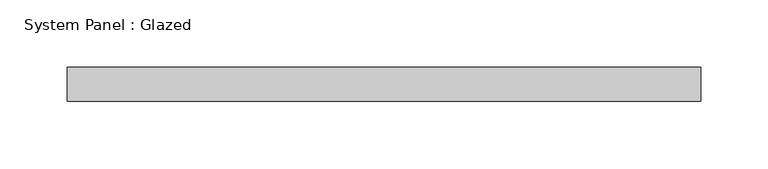
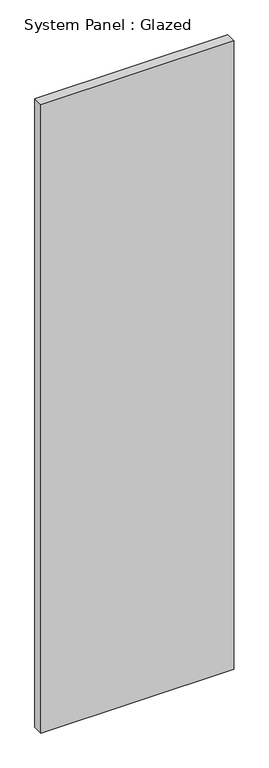
"""IFC4 building model written with IfcOpenShell, lengths in millimetres: plate geometry, System Panel : Glazed."""

from ifc_helpers import new_model, si_unit, origin, origin_with_axes, place, context, project, spatial, polyline, outline, extrude, source, transform, mapped, element, save


def system_panel_glazed_4848e608(model_context):
    return source(origin(), model_context, "Body", "SweptSolid", [
        extrude(outline(polyline([(235.7662867, 19.05), (-235.7662867, 19.05), (-235.7662867, 44.45), (235.7662867, 44.45), (235.7662867, 19.05)])), origin_with_axes(), (0.0, 0.0, 1.0), 1625.6),
    ])


if __name__ == "__main__":
    model = new_model("IFC4")
    model_context = context("Model", 3, world=origin())
    ifc_project = project(units=[si_unit("LENGTHUNIT", "METRE", prefix="MILLI")], contexts=[model_context])
    site = spatial("IfcSite", under=ifc_project)
    building = spatial("IfcBuilding", under=site)
    placement = place(None, origin())
    system_panel_glazed_shape = system_panel_glazed_4848e608(model_context)
    element("IfcPlate", 1, ObjectType="System Panel : Glazed", at=placement, inside=building, context=model_context, shape_type="MappedRepresentation", body=[
        mapped(system_panel_glazed_shape, transform((0.0, 0.0, 0.0), x_axis=(1.0, 0.0, 0.0), y_axis=(0.0, 1.0, 0.0), z_axis=(0.0, 0.0, 1.0))),
    ])
    save(model, "model.ifc")

# Revit data of these elements
# Type "System Panel : Glazed"
#   Construction Type Id = "GSP4R"
#   Analytic Construction = "1/8 in Pilkington single glazing"
#   Visual Light Transmittance = 0.9
#   Solar Heat Gain Coefficient = 0.86
#   Heat Transfer Coefficient (U) = 1.18115 BTU/(h·ft²·°F)
# Element 1 (IfcPlate, "System Panel : Glazed")
#   Materials on its faces: "Glass"
# Materials
#   "Glass": class "Glass", colour RGB 0 128 192, transparency 0.75, Description = "Soda Lime Glass", Cost = 0
